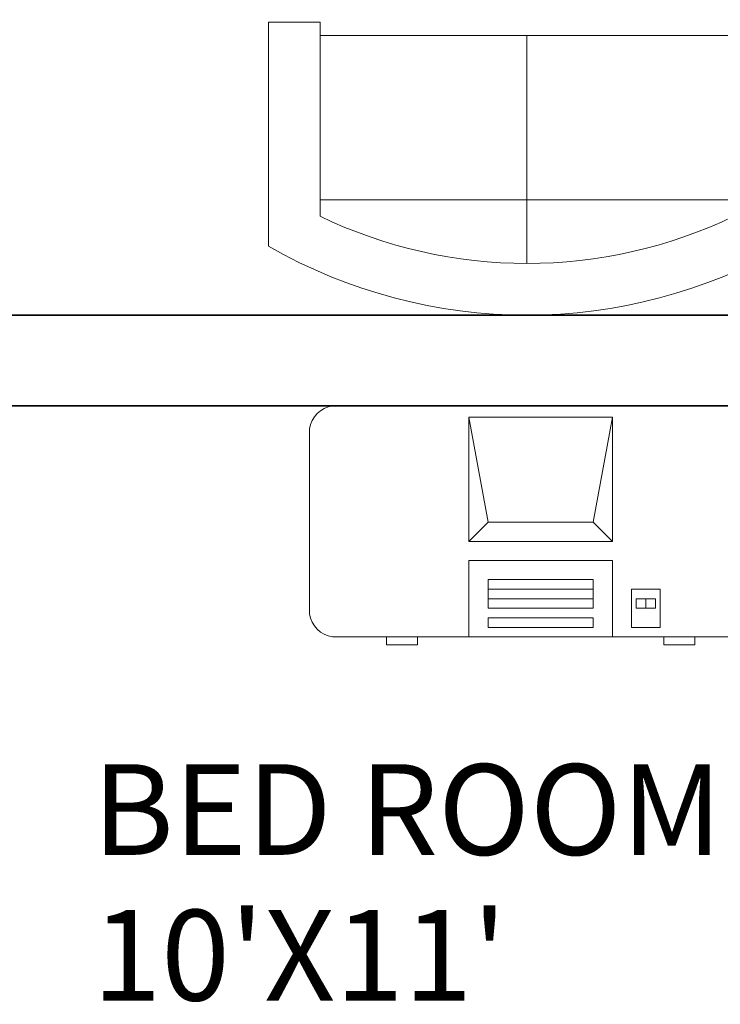
# Model space of a CAD drawing. Units: inches. Extents: x 4159 to 4826, y 299 to 1026.
# Tile 19 of 37: x 4376 to 4423, y 494 to 559. Entities that reach past the tile are written whole.
import ezdxf

# ---------------------------------------------------------------- set-up
doc = ezdxf.new("R2010")
doc.units = ezdxf.units.IN
for name, color, linetype, lineweight in [('A-ANNO-DIMS', 2, 'Continuous', 18), ('A-AREA-IDEN', 7, 'Continuous', 18), ('A-EQPM', 8, 'Continuous', 13), ('A-FURN', 8, 'Continuous', 18), ('A-WALL', 7, 'Continuous', 35)]:
    doc.layers.add(name, color=color, linetype=linetype, lineweight=lineweight)
doc.styles.get("Standard").update_dxf_attribs({"font": 'arial.ttf'})
doc.dimstyles.get("Standard").update_dxf_attribs({"dimtxt": 0.18, "dimasz": 0.18, "dimexe": 0.18, "dimexo": 0.0625, "dimgap": 0.09, "dimtad": 0, "dimtih": 1, "dimtoh": 1, "dimdec": 4, "dimzin": 0, "dimdsep": 46, "dimtxsty": 'Standard', "dimcen": 0.09, "dimadec": 0, "dimazin": 0, "dimtfac": 1, "dimtdec": 4, "dimtofl": 0, "dimtmove": 0, "dimatfit": 3, "dimfxl": 1, "dimtolj": 1, "dimtzin": 0, "dimarcsym": 0})

# ---------------------------------------------------------------- blocks, each defined once
blk = doc.blocks.new('Sofa - Roundback Loveseat 5 ft.')
for p, q in [((0, -32.44198), (0, -5.99998)), ((-24, -33.99998), (-24, -11.46958)), ((24.00004, -33.99998), (24.00004, -11.46958)), ((-23.9998, -13.38178), (23.99986, -13.38178)), ((-24, -32.44198), (24.00004, -32.44198))]:
    blk.add_line(p, q)
for points in [[(-24, -33.99998), (-30, -33.99998), (-30, -7.99998)], [(30.00004, -7.99998), (30.00004, -33.99998), (24.00004, -33.99998)]]:
    blk.add_lwpolyline(points)
for centre, radius, start, end in [((0, -60.24998), 60.24998, 60.13715, 119.8628), ((0, -61.38438), 55.38444, 64.32083, 115.6792)]:
    blk.add_arc(centre, radius, start, end)
blk = doc.blocks.new('Desk - 30 x 60 in.')
for p, q in [((-26.999995, 0), (26.999995, 0)), ((-29.999995, -27), (-29.999995, -3)), ((29.999995, -3), (29.999995, -27)), ((26.999995, -30), (-26.999995, -30)), ((-20.000005, -30), (-20.000005, -31)), ((-16.000005, -31), (-16.000005, -30)), ((15.999995, -31), (15.999995, -30)), ((19.999995, -30), (19.999995, -31)), ((-20.000005, -31), (-16.000005, -31)), ((19.999995, -31), (15.999995, -31))]:
    blk.add_line(p, q)
for centre, start, end in [((-26.499995, -3.5), 98.1301, 171.8699), ((26.499995, -3.5), 8.130102, 81.8699), ((-26.499995, -26.5), 188.1301, 261.8699), ((26.499995, -26.5), 278.1301, 351.8699)]:
    blk.add_arc(centre, 3.535534, start, end)
blk = doc.blocks.new('Computer Terminal')
for p, q in [((-10, 11.5), (5, 11.5)), ((-8, 0.5), (-10, 11.5)), ((-10, -1.5), (-10, 11.5)), ((5, 11.5), (3, 0.5)), ((5, 11.5), (5, -1.5)), ((-10, -1.5), (-8, 0.5)), ((3, 0.5), (-8, 0.5)), ((3, 0.5), (5, -1.5)), ((5, -1.5), (-10, -1.5)), ((-10, -11.5), (-10, -3.5)), ((-10, -3.5), (5, -3.5)), ((5, -3.5), (5, -11.5)), ((-8, -5.5), (-8, -8.5)), ((3, -5.5), (-8, -5.5)), ((3, -8.5), (3, -5.5)), ((3, -6.5), (-8, -6.5)), ((10, -6.5), (7, -6.5)), ((7, -6.5), (7, -10.5)), ((10, -10.5), (10, -6.5)), ((-8, -7.5), (3, -7.5)), ((9.5, -7.5), (7.5, -7.5)), ((7.5, -7.5), (7.5, -8.5)), ((8.5, -7.5), (8.5, -8.5)), ((9.5, -8.5), (9.5, -7.5)), ((-8, -8.5), (3, -8.5)), ((7.5, -8.5), (9.5, -8.5)), ((-8, -9.5), (-8, -10.5)), ((3, -9.5), (-8, -9.5)), ((3, -10.5), (3, -9.5)), ((-8, -10.5), (3, -10.5)), ((7, -10.5), (10, -10.5)), ((5, -11.5), (-10, -11.5))]:
    blk.add_line(p, q)
blk = doc.blocks.new('*D44')
at = {"layer": 'A-ANNO-DIMS', "color": 0, "lineweight": -2, "transparency": 16777216}
for p, q in [((4287.263, 963.093), (4158.88, 963.093)), ((4159.06, 962.913), (4159.06, 647.826)), ((4159.06, 332.375), (4159.06, 647.462)), ((4447.248, 332.195), (4158.88, 332.195))]:
    blk.add_line(p, q, dxfattribs=at)
at = {"layer": 'A-ANNO-DIMS', "color": 0, "transparency": 16777216}
for points in [[(4159.03, 962.913), (4159.09, 962.913), (4159.06, 963.093)], [(4159.03, 332.375), (4159.09, 332.375), (4159.06, 332.195)]]:
    blk.add_solid(points, dxfattribs=at)
at = {"layer": 'Defpoints', "color": 0, "transparency": 16777216}
for p in [(4287.326, 963.093), (4159.06, 332.195), (4447.31, 332.195)]:
    blk.add_point(p, dxfattribs=at)
at = {"layer": 'A-ANNO-DIMS', "color": 0, "transparency": 16777216, "insert": (4159.06, 647.644), "char_height": 0.18, "attachment_point": 5}
blk.add_mtext('\\A1;630.9', dxfattribs=at)

msp = doc.modelspace()

# ---------------------------------------------------------------- linework, layer by layer
at = {"layer": 'A-WALL'}
for p, q in [((4447.31, 539.254), (4369.31, 539.254)), ((4447.31, 533.254), (4369.31, 533.254))]:
    msp.add_line(p, q, dxfattribs=at)

# ---------------------------------------------------------------- block references
at = {"layer": 'A-EQPM', "xscale": 0.6328414688201627, "yscale": 0.6328414688201627, "zscale": 0.6328414688201627}
msp.add_blockref('Computer Terminal', (4412.328, 525.235), dxfattribs=at)
at = {"layer": 'A-FURN', "xscale": 0.5700533147329089, "yscale": 0.5700533147329089, "zscale": 0.5700533147329089, "rotation": 180}
msp.add_blockref('Sofa - Roundback Loveseat 5 ft.', (4409.841, 539.254), dxfattribs=at)
at = {"layer": 'A-FURN', "xscale": 0.5098837128326598, "yscale": 0.5098837128326598, "zscale": 0.5098837128326598}
msp.add_blockref('Desk - 30 x 60 in.', (4410.746, 533.254), dxfattribs=at)

# ---------------------------------------------------------------- texts
at = {"layer": 'A-AREA-IDEN'}
for s, p in [('BED ROOM', (4381.096, 503.539)), ("10'X11'", (4381.096, 493.9))]:
    msp.add_text(s, height=6, dxfattribs=at).set_placement(p)

# ---------------------------------------------------------------- dimensions: what is measured, and where the dimension line sits
at = {"layer": 'A-ANNO-DIMS'}
dim = msp.add_linear_dim(base=(4159.06, 332.195), p1=(4287.326, 963.093), p2=(4447.31, 332.195), angle=90, dimstyle='Standard', override={"dimdec": 1, "dimlfac": 1, "dimrnd": 0, "dimzin": 0, "dimdsep": 46, "dimlunit": 2}, dxfattribs=at)
dim.commit()
dim.dimension.update_dxf_attribs({"geometry": '*D44', "text_midpoint": (4159.06, 647.644)})

doc.saveas('drawing.dxf')
